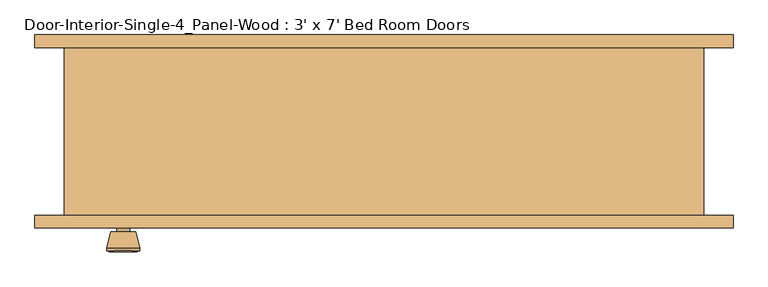
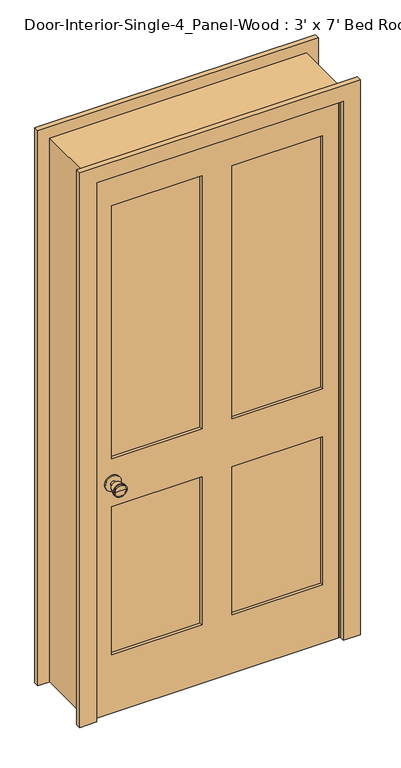
"""IFC4 building model written with IfcOpenShell, lengths in millimetres: door geometry, Door-Interior-Single-4_Panel-Wood : 3' x 7' Bed Room Doors."""

from ifc_helpers import new_model, si_unit, point, frame, frame_2d, origin, place, context, project, spatial, polyline, circle_curve, trimmed, segment, composite_curve, outline, extrude, faceted_brep, source, transform, mapped, element, save
from ifc_brep_helpers import plane_surface, cylinder_surface, revolved_surface, advanced_brep


def door_interior_single_4_panel_wood_3_x_7_bed_room_doors_7969a7cd(model_context):
    return source(origin(), model_context, "Body", "SolidModel", [
        advanced_brep(
        [(-393.7, -82.9, 914.4), (-403.7, -82.9, 914.4), (-383.7, -82.9, 914.4), (-373.2241324, -33.9, 914.4), (-414.1758676, -33.9, 914.4), (-393.7, -33.9, 914.4), (-368.7, -35.7278681, 914.4), (-418.7, -35.7278681, 914.4), (-368.7, -39.1915463, 914.4), (-418.7, -39.1915463, 914.4), (-375.063764, -63.9, 914.4), (-412.336236, -63.9, 914.4), (-383.7, -63.9, 914.4), (-403.7, -63.9, 914.4)],
        [
            (0, 1),
            (1, 2, circle_curve(frame((-393.7, -82.9, 914.4), z_axis=(0.0, -1.0, 0.0), x_axis=(-1.0, 0.0, 0.0)), 10.0)),
            (2, 0),
            (2, 1, circle_curve(frame((-393.7, -82.9, 914.4), z_axis=(0.0, -1.0, 0.0), x_axis=(-1.0, 0.0, 0.0)), 10.0)),
            (3, 4, circle_curve(frame((-393.7, -33.9, 914.4), z_axis=(0.0, 1.0, 0.0), x_axis=(-1.0, 0.0, 0.0)), 20.4758676)),
            (4, 5),
            (5, 3),
            (4, 3, circle_curve(frame((-393.7, -33.9, 914.4), z_axis=(0.0, 1.0, 0.0), x_axis=(-1.0, 0.0, 0.0)), 20.4758676)),
            (6, 7, circle_curve(frame((-393.7, -35.7278681, 914.4), z_axis=(0.0, 1.0, 0.0), x_axis=(-1.0, 0.0, 0.0)), 25.0)),
            (7, 4),
            (3, 6),
            (7, 6, circle_curve(frame((-393.7, -35.7278681, 914.4), z_axis=(0.0, 1.0, 0.0), x_axis=(-1.0, 0.0, 0.0)), 25.0)),
            (8, 9, circle_curve(frame((-393.7, -39.1915463, 914.4), z_axis=(0.0, 1.0, 0.0), x_axis=(-1.0, 0.0, 0.0)), 25.0)),
            (9, 7),
            (6, 8),
            (9, 8, circle_curve(frame((-393.7, -39.1915463, 914.4), z_axis=(0.0, 1.0, 0.0), x_axis=(-1.0, 0.0, 0.0)), 25.0)),
            (10, 11, circle_curve(frame((-393.7, -63.9, 914.4), z_axis=(0.0, 1.0, 0.0), x_axis=(-1.0, 0.0, 0.0)), 18.636236)),
            (11, 9),
            (8, 10),
            (11, 10, circle_curve(frame((-393.7, -63.9, 914.4), z_axis=(0.0, 1.0, 0.0), x_axis=(-1.0, 0.0, 0.0)), 18.636236)),
            (12, 13, circle_curve(frame((-393.7, -63.9, 914.4), z_axis=(0.0, 1.0, 0.0), x_axis=(-1.0, 0.0, 0.0)), 10.0)),
            (13, 11),
            (10, 12),
            (13, 12, circle_curve(frame((-393.7, -63.9, 914.4), z_axis=(0.0, 1.0, 0.0), x_axis=(-1.0, 0.0, 0.0)), 10.0)),
            (1, 13),
            (12, 2),
        ],
        [
            plane_surface(frame((-393.7, -82.9, 914.4), z_axis=(0.0, -1.0, 0.0), x_axis=(-1.0, 0.0, 0.0))),
            plane_surface(frame((-393.7, -33.9, 914.4), z_axis=(0.0, 1.0, 0.0), x_axis=(-1.0, 0.0, 0.0))),
            revolved_surface(polyline([(-414.1758676, -33.9, 914.4), (-418.7, -35.7278681, 914.4)]), (-393.7, -82.9, 914.4), (0.0, -1.0, 0.0)),
            cylinder_surface(frame((-393.7, -82.9, 914.4), z_axis=(0.0, -1.0, 0.0), x_axis=(-1.0, 0.0, 0.0)), 25.0),
            revolved_surface(polyline([(-418.7, -39.1915463, 914.4), (-412.336236, -63.9, 914.4)]), (-393.7, -82.9, 914.4), (0.0, -1.0, 0.0)),
            plane_surface(frame((-393.7, -63.9, 914.4), z_axis=(0.0, -1.0, 0.0), x_axis=(-1.0, 0.0, 0.0))),
            cylinder_surface(frame((-393.7, -82.9, 914.4), z_axis=(0.0, -1.0, 0.0), x_axis=(-1.0, 0.0, 0.0)), 10.0),
        ],
        [
            (0, [[1, 2, 3]]),
            (0, [[-3, 4, -1]]),
            (1, [[5, 6, 7]]),
            (1, [[8, -7, -6]]),
            (2, [[9, 10, -5, 11]]),
            (2, [[12, -11, -8, -10]]),
            (3, [[13, 14, -9, 15]]),
            (3, [[16, -15, -12, -14]]),
            (4, [[17, 18, -13, 19]]),
            (4, [[20, -19, -16, -18]]),
            (5, [[21, 22, -17, 23]]),
            (5, [[24, -23, -20, -22]]),
            (6, [[-2, 25, -21, 26]]),
            (6, [[-4, -26, -24, -25]]),
        ],
    ),
        extrude(outline(composite_curve([segment(trimmed(circle_curve(frame_2d((914.4, -393.7)), 30.0), [point((914.4, -423.7))], [point((914.4, -363.7))], False, "CARTESIAN"), True, "CONTINUOUS"), segment(trimmed(circle_curve(frame_2d((914.4, -393.7)), 30.0), [point((914.4, -363.7))], [point((914.4, -423.7))], False, "CARTESIAN"), True, "CONTINUOUS")], self_intersect=False)), frame((0.0, -88.9, 0.0), z_axis=(0.0, 1.0, 0.0), x_axis=(0.0, 0.0, 1.0)), (0.0, 0.0, 1.0), 6.0),
        advanced_brep(
        [(-393.7, -129.825, 914.4), (-383.7, -129.825, 914.4), (-403.7, -129.825, 914.4), (-373.2241324, -178.825, 914.4), (-393.7, -178.825, 914.4), (-414.1758676, -178.825, 914.4), (-368.7, -176.9971319, 914.4), (-418.7, -176.9971319, 914.4), (-368.7, -173.5334537, 914.4), (-418.7, -173.5334537, 914.4), (-375.063764, -148.825, 914.4), (-412.336236, -148.825, 914.4), (-383.7, -148.825, 914.4), (-403.7, -148.825, 914.4)],
        [
            (0, 1),
            (1, 2, circle_curve(frame((-393.7, -129.825, 914.4), z_axis=(0.0, 1.0, 0.0), x_axis=(-1.0, 0.0, 0.0)), 10.0)),
            (2, 0),
            (2, 1, circle_curve(frame((-393.7, -129.825, 914.4), z_axis=(0.0, 1.0, 0.0), x_axis=(-1.0, 0.0, 0.0)), 10.0)),
            (3, 4),
            (4, 5),
            (5, 3, circle_curve(frame((-393.7, -178.825, 914.4), z_axis=(0.0, -1.0, 0.0), x_axis=(-1.0, 0.0, 0.0)), 20.4758676)),
            (3, 5, circle_curve(frame((-393.7, -178.825, 914.4), z_axis=(0.0, -1.0, 0.0), x_axis=(-1.0, 0.0, 0.0)), 20.4758676)),
            (6, 3),
            (5, 7),
            (7, 6, circle_curve(frame((-393.7, -176.9971319, 914.4), z_axis=(0.0, -1.0, 0.0), x_axis=(-1.0, 0.0, 0.0)), 25.0)),
            (6, 7, circle_curve(frame((-393.7, -176.9971319, 914.4), z_axis=(0.0, -1.0, 0.0), x_axis=(-1.0, 0.0, 0.0)), 25.0)),
            (8, 6),
            (7, 9),
            (9, 8, circle_curve(frame((-393.7, -173.5334537, 914.4), z_axis=(0.0, -1.0, 0.0), x_axis=(-1.0, 0.0, 0.0)), 25.0)),
            (8, 9, circle_curve(frame((-393.7, -173.5334537, 914.4), z_axis=(0.0, -1.0, 0.0), x_axis=(-1.0, 0.0, 0.0)), 25.0)),
            (10, 8),
            (9, 11),
            (11, 10, circle_curve(frame((-393.7, -148.825, 914.4), z_axis=(0.0, -1.0, 0.0), x_axis=(-1.0, 0.0, 0.0)), 18.636236)),
            (10, 11, circle_curve(frame((-393.7, -148.825, 914.4), z_axis=(0.0, -1.0, 0.0), x_axis=(-1.0, 0.0, 0.0)), 18.636236)),
            (12, 10),
            (11, 13),
            (13, 12, circle_curve(frame((-393.7, -148.825, 914.4), z_axis=(0.0, -1.0, 0.0), x_axis=(-1.0, 0.0, 0.0)), 10.0)),
            (12, 13, circle_curve(frame((-393.7, -148.825, 914.4), z_axis=(0.0, -1.0, 0.0), x_axis=(-1.0, 0.0, 0.0)), 10.0)),
            (1, 12),
            (13, 2),
        ],
        [
            plane_surface(frame((-393.7, -129.825, 914.4), z_axis=(0.0, 1.0, 0.0), x_axis=(-1.0, 0.0, 0.0))),
            plane_surface(frame((-393.7, -178.825, 914.4), z_axis=(0.0, -1.0, 0.0), x_axis=(-1.0, 0.0, 0.0))),
            revolved_surface(polyline([(-414.1758676, -178.825, 914.4), (-418.7, -176.9971319, 914.4)]), (-393.7, -129.825, 914.4), (0.0, 1.0, 0.0)),
            cylinder_surface(frame((-393.7, -129.825, 914.4), z_axis=(0.0, 1.0, 0.0), x_axis=(-1.0, 0.0, 0.0)), 25.0),
            revolved_surface(polyline([(-418.7, -173.5334537, 914.4), (-412.336236, -148.825, 914.4)]), (-393.7, -129.825, 914.4), (0.0, 1.0, 0.0)),
            plane_surface(frame((-393.7, -148.825, 914.4), z_axis=(0.0, 1.0, 0.0), x_axis=(-1.0, 0.0, 0.0))),
            cylinder_surface(frame((-393.7, -129.825, 914.4), z_axis=(0.0, 1.0, 0.0), x_axis=(-1.0, 0.0, 0.0)), 10.0),
        ],
        [
            (0, [[1, 2, 3]]),
            (0, [[-3, 4, -1]]),
            (1, [[5, 6, 7]]),
            (1, [[-6, -5, 8]]),
            (2, [[9, -7, 10, 11]]),
            (2, [[-10, -8, -9, 12]]),
            (3, [[13, -11, 14, 15]]),
            (3, [[-14, -12, -13, 16]]),
            (4, [[17, -15, 18, 19]]),
            (4, [[-18, -16, -17, 20]]),
            (5, [[21, -19, 22, 23]]),
            (5, [[-22, -20, -21, 24]]),
            (6, [[25, -23, 26, -2]]),
            (6, [[-26, -24, -25, -4]]),
        ],
    ),
        extrude(outline(composite_curve([segment(trimmed(circle_curve(frame_2d((914.4, -393.7)), 30.0), [point((914.4, -423.7))], [point((914.4, -363.7))], False, "CARTESIAN"), True, "CONTINUOUS"), segment(trimmed(circle_curve(frame_2d((914.4, -393.7)), 30.0), [point((914.4, -363.7))], [point((914.4, -423.7))], False, "CARTESIAN"), True, "CONTINUOUS")], self_intersect=False)), frame((0.0, -129.825, 0.0), z_axis=(0.0, 1.0, 0.0), x_axis=(0.0, 0.0, 1.0)), (0.0, 0.0, 1.0), 6.0),
        faceted_brep([(482.6, -123.825, 0.0), (457.2, -123.825, 0.0), (457.2, -88.9, 0.0), (444.5, -88.9, 0.0), (444.5, -53.975, 0.0), (457.2, -53.975, 0.0), (457.2, 130.175, 0.0), (482.6, 130.175, 0.0), (482.6, 130.175, 2159.0), (482.6, -123.825, 2159.0), (457.2, 130.175, 2133.6), (-457.2, 130.175, 2133.6), (-457.2, 130.175, 0.0), (-482.6, 130.175, 0.0), (-482.6, 130.175, 2159.0), (457.2, -53.975, 2133.6), (444.5, -53.975, 2120.9), (-444.5, -53.975, 2120.9), (-444.5, -53.975, 0.0), (-457.2, -53.975, 0.0), (-457.2, -53.975, 2133.6), (444.5, -88.9, 2120.9), (457.2, -88.9, 2133.6), (-457.2, -88.9, 2133.6), (-457.2, -88.9, 0.0), (-444.5, -88.9, 0.0), (-444.5, -88.9, 2120.9), (457.2, -123.825, 2133.6), (-482.6, -123.825, 2159.0), (-482.6, -123.825, 0.0), (-457.2, -123.825, 0.0), (-457.2, -123.825, 2133.6)], [[[0, 1, 2, 3, 4, 5, 6, 7]], [[7, 8, 9, 0]], [[6, 10, 11, 12, 13, 14, 8, 7]], [[5, 15, 10, 6]], [[4, 16, 17, 18, 19, 20, 15, 5]], [[3, 21, 16, 4]], [[2, 22, 23, 24, 25, 26, 21, 3]], [[1, 27, 22, 2]], [[0, 9, 28, 29, 30, 31, 27, 1]], [[8, 14, 28, 9]], [[15, 20, 11, 10]], [[21, 26, 17, 16]], [[27, 31, 23, 22]], [[29, 13, 12, 19, 18, 25, 24, 30]], [[14, 13, 29, 28]], [[20, 19, 12, 11]], [[26, 25, 18, 17]], [[31, 30, 24, 23]]]),
        extrude(outline(polyline([(2133.6, -457.2), (0.0, -457.2), (0.0, 457.2), (2133.6, 457.2), (2133.6, -457.2)]), holes=[polyline([(2014.5375, 57.15), (2014.5375, 396.875), (1009.65, 396.875), (1009.65, 57.15), (2014.5375, 57.15)]), polyline([(1009.65, -57.15), (1009.65, -396.875), (2014.5375, -396.875), (2014.5375, -57.15), (1009.65, -57.15)]), polyline([(819.15, 57.15), (819.15, 396.875), (231.775, 396.875), (231.775, 57.15), (819.15, 57.15)]), polyline([(231.775, -57.15), (231.775, -396.875), (819.15, -396.875), (819.15, -57.15), (231.775, -57.15)])]), frame((0.0, -123.825, 0.0), z_axis=(0.0, 1.0, 0.0), x_axis=(0.0, 0.0, 1.0)), (0.0, 0.0, 1.0), 34.925),
        extrude(outline(polyline([(396.875, -100.5416667), (396.875, -112.1833333), (57.15, -112.1833333), (57.15, -100.5416667), (396.875, -100.5416667)])), frame((0.0, 0.0, 1009.65), z_axis=(0.0, 0.0, 1.0), x_axis=(1.0, 0.0, 0.0)), (0.0, 0.0, 1.0), 1004.8875),
        extrude(outline(polyline([(-57.15, -100.5416667), (-57.15, -112.1833333), (-396.875, -112.1833333), (-396.875, -100.5416667), (-57.15, -100.5416667)])), frame((0.0, 0.0, 1009.65), z_axis=(0.0, 0.0, 1.0), x_axis=(1.0, 0.0, 0.0)), (0.0, 0.0, 1.0), 1004.8875),
        extrude(outline(polyline([(396.875, -100.5416667), (396.875, -112.1833333), (57.15, -112.1833333), (57.15, -100.5416667), (396.875, -100.5416667)])), frame((0.0, 0.0, 231.775), z_axis=(0.0, 0.0, 1.0), x_axis=(1.0, 0.0, 0.0)), (0.0, 0.0, 1.0), 587.375),
        extrude(outline(polyline([(-57.15, -100.5416667), (-57.15, -112.1833333), (-396.875, -112.1833333), (-396.875, -100.5416667), (-57.15, -100.5416667)])), frame((0.0, 0.0, 231.775), z_axis=(0.0, 0.0, 1.0), x_axis=(1.0, 0.0, 0.0)), (0.0, 0.0, 1.0), 587.375),
        extrude(outline(polyline([(0.0, 527.05), (2203.45, 527.05), (2203.45, -527.05), (0.0, -527.05), (0.0, -463.55), (2139.95, -463.55), (2139.95, 463.55), (0.0, 463.55), (0.0, 527.05)])), frame((0.0, -142.875, 0.0), z_axis=(0.0, 1.0, 0.0), x_axis=(0.0, 0.0, 1.0)), (0.0, 0.0, 1.0), 19.05),
        extrude(outline(polyline([(0.0, 527.05), (2203.45, 527.05), (2203.45, -527.05), (0.0, -527.05), (0.0, -463.55), (2139.95, -463.55), (2139.95, 463.55), (0.0, 463.55), (0.0, 527.05)])), frame((0.0, 130.175, 0.0), z_axis=(0.0, 1.0, 0.0), x_axis=(0.0, 0.0, 1.0)), (0.0, 0.0, 1.0), 19.05),
    ])


if __name__ == "__main__":
    model = new_model("IFC4")
    model_context = context("Model", 3, world=origin())
    ifc_project = project(units=[si_unit("LENGTHUNIT", "METRE", prefix="MILLI")], contexts=[model_context])
    site = spatial("IfcSite", under=ifc_project)
    building = spatial("IfcBuilding", under=site)
    placement = place(None, origin())
    door_interior_single_4_panel_wood_3_x_7_bed_room_doors_shape = door_interior_single_4_panel_wood_3_x_7_bed_room_doors_7969a7cd(model_context)
    element("IfcDoor", 1, ObjectType="Door-Interior-Single-4_Panel-Wood : 3' x 7' Bed Room Doors", at=placement, inside=building, context=model_context, shape_type="MappedRepresentation", body=[
        mapped(door_interior_single_4_panel_wood_3_x_7_bed_room_doors_shape, transform((0.0, 0.0, 0.0), x_axis=(1.0, 0.0, 0.0), y_axis=(0.0, 1.0, 0.0), z_axis=(0.0, 0.0, 1.0))),
    ])
    save(model, "model.ifc")

# Revit data of these elements
# Type "Door-Interior-Single-4_Panel-Wood : 3' x 7' Bed Room Doors"
#   Type Mark = "13"
#   Assembly Code = "C1020300"
#   Analytic Construction = "Wooden"
#   Top Rail = 0' - 4 11/16"
#   Thickness = 0' - 1 3/8"
#   Thermal Resistance (R) = 2.5876 (h·ft²·°F)/BTU
#   Swing Angle [instance default] = 90.00°
#   Stiles = 0' - 2 3/8"
#   Rough Width = 3' - 2"
#   Rough Height = 7' - 1"
#   Mullion = 0' - 4 1/2"
#   Lock Rail = 0' - 7 1/2"
#   Height = 7' - 0"
#   Width = 3' - 0"
#   Heat Transfer Coefficient (U) = 0.3865 BTU/(h·ft²·°F)
#   Bottom Rail = 0' - 9 1/8"
#   Trim Material = Cherry
#   Panel Material = Cherry
#   Frame Material = Cherry
#   Door Handle Material = Aluminum
#   Visual Light Transmittance = 0
#   Solar Heat Gain Coefficient = 0
#   Wall Closure = (empty or 0)
#   Function = (empty or 0)
# Element 1 (IfcDoor, "Door-Interior-Single-4_Panel-Wood : 3' x 7' Bed Room Doors")
#   Materials on its faces: "Cherry", "Aluminum"
# Materials
#   "Cherry": class "Wood", colour RGB 226 177 128, transparency 0, Description = "Prunus Serotina", Cost = 0
#   "Aluminum": class "Metal", colour RGB 247 247 247, transparency 0, Description = "Aluminum 6061", Cost = 0
